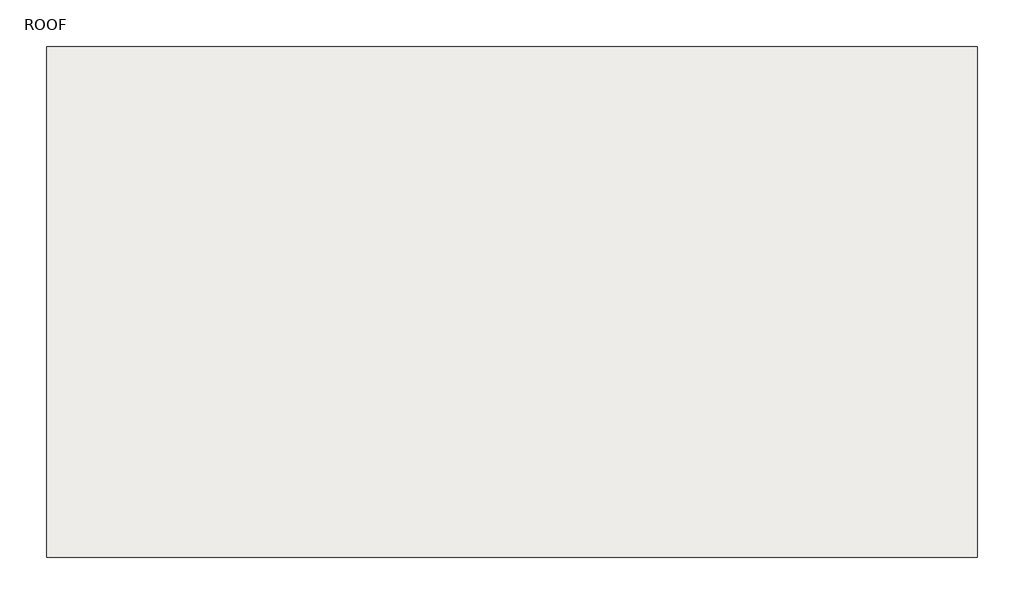
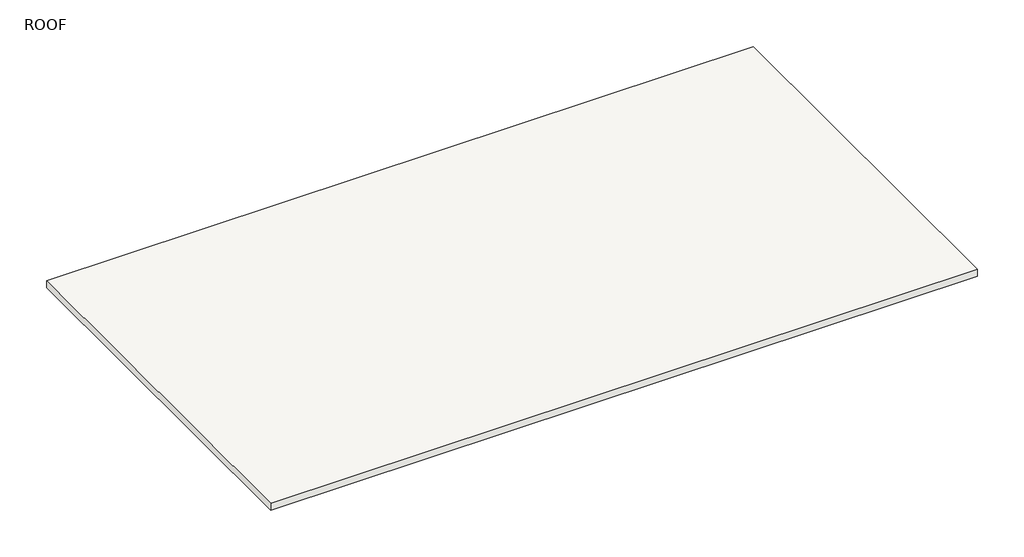
# One storey: 1 slab.
"""IFC4 building model written with IfcOpenShell, lengths in millimetres."""

from ifc_helpers import new_model, si_unit, frame, origin, place, context, project, spatial, polyline, outline, extrude, element, save

model = new_model("IFC4")

# Units and contexts
model_context = context("Model", 3, world=origin())
ifc_project = project(units=[si_unit("LENGTHUNIT", "METRE", prefix="MILLI")], contexts=[model_context])

# Site, building, storey
site = spatial("IfcSite", under=ifc_project)
building = spatial("IfcBuilding", under=site)
storey = spatial("IfcBuildingStorey", under=building, Name="ROOF", Elevation=9160.6695361)

# Slab
placement = place(None, origin())
element("IfcSlab", 1, ObjectType="Generic 150mm", at=placement, inside=storey, context=model_context, shape_type="SweptSolid", body=[
    extrude(outline(polyline([(6740.1178986, 5013.6018891), (-7325.2166703, 5013.6018891), (-7325.2166703, 12732.936458), (6740.1178986, 12732.936458), (6740.1178986, 5013.6018891)])), frame((0.0, 0.0, 9010.6695361), z_axis=(0.0, 0.0, 1.0), x_axis=(1.0, 0.0, 0.0)), (0.0, 0.0, 1.0), 150.0),
])

save(model, "model.ifc")

# Revit data of these elements
# Type "Generic 150mm"
#   Function = 0
#   Layers, outside or top first: 150 mm "Render, Tan, Textured" (function 1)
# Element 1 (IfcSlab, "Generic 150mm")
#   Height Offset From Level = 0 mm
#   Phase Created = New Construction
#   Materials on its faces: "Render, Tan, Textured", "Wood Planks"
# Materials
#   "Render, Tan, Textured": class "Generic", colour RGB 196 158 130, transparency 0, Description = "physical material", Cost = 0
#   "Wood Planks": class "Wood", colour RGB 193 160 115, transparency 0, Description = "Physical material.", Cost = 0
